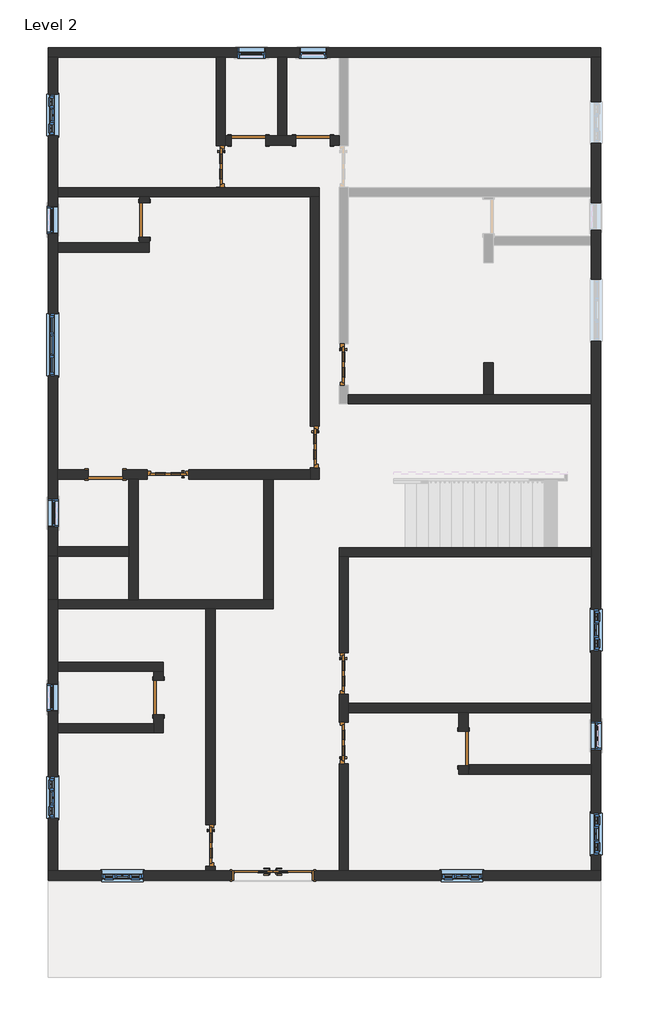
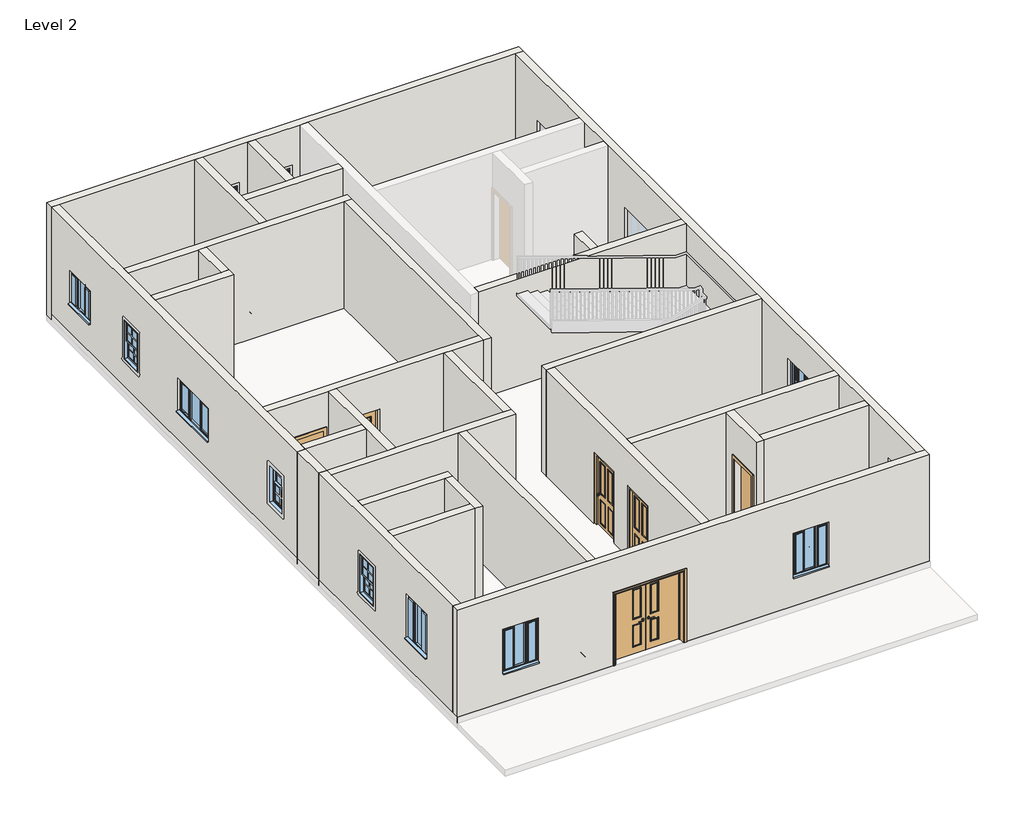
# One storey, part 1 of 3: 29 walls, 14 doors, 13 windows.
"""IFC4 building model written with IfcOpenShell, lengths in millimetres."""

from ifc_helpers import new_model, si_unit, frame, origin, place, context, project, spatial, polyline, outline, extrude, faceted_brep, transform, mapped, element, save
from components import door_2817e3e8, door_51b0c682, doors_intdbl_3_1810x2110mm_301b02ef, doors_intdbl_3_1810x2110mm_13513f6f, door_fadea3f2, door_53b1b562, window_679d2811, windows_tpl_plain_1360x910mm_84993ef1, windows_tpl_w_glazing_cross_bars_910x1210mm_e0b59135, windows_tpl_w_glazing_cross_bars_910x910mm_4aa0f884

model = new_model("IFC4")

# Units and contexts
model_context = context("Model", 3, world=origin())
ifc_project = project(units=[si_unit("LENGTHUNIT", "METRE", prefix="MILLI")], contexts=[model_context])

# Site, building, storey
site = spatial("IfcSite", under=ifc_project)
building = spatial("IfcBuilding", under=site)
storey = spatial("IfcBuildingStorey", under=building, Name="Level 2", Elevation=3048.0)

# Doors
placement = place(None, origin())
door_shape = door_2817e3e8(model_context)
element("IfcDoor", 1, ObjectType="Doors_ExtSgl_2 : 2'x7\"", at=placement, inside=storey, context=model_context, shape_type="MappedRepresentation", body=[
    mapped(door_shape, transform((-2349.4166288, 6357.8803322, 3048.0), x_axis=(0.0, -1.0, 0.0), y_axis=(1.0, 0.0, 0.0), z_axis=(0.0, 0.0, 1.0))),
])
element("IfcDoor", 2, ObjectType="Doors_ExtSgl_2 : 2'x7\"", at=placement, inside=storey, context=model_context, shape_type="MappedRepresentation", body=[
    mapped(door_shape, transform((-286.4451949, 208.0340986, 3048.0), x_axis=(0.0, -1.0, 0.0), y_axis=(1.0, 0.0, 0.0), z_axis=(0.0, 0.0, 1.0))),
])
element("IfcDoor", 3, ObjectType="Doors_ExtSgl_2 : 2'x7\"", at=placement, inside=storey, context=model_context, shape_type="MappedRepresentation", body=[
    mapped(door_shape, transform((348.5548051, -6285.6488489, 3048.0), x_axis=(0.0, 1.0, 0.0), y_axis=(-1.0, 0.0, 0.0), z_axis=(0.0, 0.0, 1.0))),
])
element("IfcDoor", 4, ObjectType="Doors_ExtSgl_2 : 2'x7\"", at=placement, inside=storey, context=model_context, shape_type="MappedRepresentation", body=[
    mapped(door_shape, transform((-2575.1220989, -8536.1734342, 3048.0), x_axis=(0.0, -1.0, 0.0), y_axis=(1.0, 0.0, 0.0), z_axis=(0.0, 0.0, 1.0))),
])
door_2_shape = door_51b0c682(model_context)
element("IfcDoor", 5, ObjectType="Doors_ExtSgl_2 : 2'x7\"", at=placement, inside=storey, context=model_context, shape_type="MappedRepresentation", body=[
    mapped(door_2_shape, transform((348.5548051, -4761.6488489, 3048.0), x_axis=(0.0, -1.0, 0.0), y_axis=(1.0, 0.0, 0.0), z_axis=(0.0, 0.0, 1.0))),
])
element("IfcDoor", 6, ObjectType="Doors_ExtSgl_2 : 2'x7\"", at=placement, inside=storey, context=model_context, shape_type="MappedRepresentation", body=[
    mapped(door_2_shape, transform((-3502.9153286, -401.5659014, 3048.0), x_axis=(-1.0, 0.0, 0.0), y_axis=(0.0, -1.0, 0.0), z_axis=(0.0, 0.0, 1.0))),
])
element("IfcDoor", 7, ObjectType="Doors_ExtSgl_2 : 2'x7\"", at=placement, inside=storey, context=model_context, shape_type="MappedRepresentation", body=[
    mapped(door_2_shape, transform((348.5548051, 2011.4340986, 3048.0), x_axis=(0.0, -1.0, 0.0), y_axis=(1.0, 0.0, 0.0), z_axis=(0.0, 0.0, 1.0))),
])
doors_intdbl_3_1810x2110mm_shape = doors_intdbl_3_1810x2110mm_301b02ef(model_context)
doors_intdbl_3_1810x2110mm_2_shape = doors_intdbl_3_1810x2110mm_13513f6f(model_context)
element("IfcDoor", 8, ObjectType="Doors_IntDbl_3 : 1810x2110mm", at=placement, inside=storey, context=model_context, shape_type="MappedRepresentation", body=[
    mapped(doors_intdbl_3_1810x2110mm_shape, transform((-1203.5220989, -9196.5734342, 3048.0), x_axis=(-1.0, 0.0, 0.0), y_axis=(0.0, -1.0, 0.0), z_axis=(0.0, 0.0, 1.0))),
    mapped(doors_intdbl_3_1810x2110mm_2_shape, transform((-1203.5220989, -9196.5734342, 3048.0), x_axis=(-1.0, 0.0, 0.0), y_axis=(0.0, -1.0, 0.0), z_axis=(0.0, 0.0, 1.0))),
])
door_3_shape = door_fadea3f2(model_context)
element("IfcDoor", 9, ObjectType="Single-Flush : 30\" x 80\"", at=placement, inside=storey, context=model_context, shape_type="MappedRepresentation", body=[
    mapped(door_3_shape, transform((-1739.8166288, 6926.3340986, 3048.0), x_axis=(1.0, 0.0, 0.0), y_axis=(0.0, 1.0, 0.0), z_axis=(0.0, 0.0, 1.0))),
])
element("IfcDoor", 10, ObjectType="Single-Flush : 30\" x 80\"", at=placement, inside=storey, context=model_context, shape_type="MappedRepresentation", body=[
    mapped(door_3_shape, transform((-4874.5153286, -401.5659014, 3048.0), x_axis=(-1.0, 0.0, 0.0), y_axis=(0.0, -1.0, 0.0), z_axis=(0.0, 0.0, 1.0))),
])
door_4_shape = door_53b1b562(model_context)
element("IfcDoor", 11, ObjectType="Single-Flush : 30\" x 80\"", at=placement, inside=storey, context=model_context, shape_type="MappedRepresentation", body=[
    mapped(door_4_shape, transform((-324.5451949, 6926.3340986, 3048.0), x_axis=(-1.0, 0.0, 0.0), y_axis=(0.0, -1.0, 0.0), z_axis=(0.0, 0.0, 1.0))),
])
element("IfcDoor", 12, ObjectType="Single-Flush : 30\" x 80\"", at=placement, inside=storey, context=model_context, shape_type="MappedRepresentation", body=[
    mapped(door_4_shape, transform((-3715.4451949, -5291.0659014, 3048.0), x_axis=(0.0, -1.0, 0.0), y_axis=(1.0, 0.0, 0.0), z_axis=(0.0, 0.0, 1.0))),
])
element("IfcDoor", 13, ObjectType="Single-Flush : 30\" x 80\"", at=placement, inside=storey, context=model_context, shape_type="MappedRepresentation", body=[
    mapped(door_4_shape, transform((2977.4548051, -6412.6488489, 3048.0), x_axis=(0.0, 1.0, 0.0), y_axis=(-1.0, 0.0, 0.0), z_axis=(0.0, 0.0, 1.0))),
])
element("IfcDoor", 14, ObjectType="Single-Flush : 30\" x 80\"", at=placement, inside=storey, context=model_context, shape_type="MappedRepresentation", body=[
    mapped(door_4_shape, transform((-4023.5839448, 5183.1303322, 3048.0), x_axis=(0.0, -1.0, 0.0), y_axis=(1.0, 0.0, 0.0), z_axis=(0.0, 0.0, 1.0))),
])

# Walls
element("IfcWall", 15, ObjectType="Generic - 4.5\" p", at=placement, inside=storey, context=model_context, shape_type="Brep", body=[
    faceted_brep([(-5928.5839448, 5687.8265658, 3048.0), (-4125.1839448, 5687.8265658, 3048.0), (-3921.9839448, 5687.8265658, 3048.0), (-388.0451949, 5687.8265658, 3048.0), (-184.8451949, 5687.8265658, 3048.0), (-184.8451949, 5687.8265658, 6096.0), (-388.0451949, 5687.8265658, 6096.0), (-3921.9839448, 5687.8265658, 6096.0), (-4125.1839448, 5687.8265658, 6096.0), (-5928.5839448, 5687.8265658, 6096.0), (-5928.5839448, 5891.0265658, 3048.0), (-5928.5839448, 5891.0265658, 6096.0), (-2451.0166288, 5891.0265658, 6096.0), (-2247.8166288, 5891.0265658, 6096.0), (-184.8451949, 5891.0265658, 6096.0), (-184.8451949, 5891.0265658, 3048.0), (-2247.8166288, 5891.0265658, 3048.0), (-2451.0166288, 5891.0265658, 3048.0)], [[[0, 1, 2, 3, 4, 5, 6, 7, 8, 9]], [[10, 11, 12, 13, 14, 15, 16, 17]], [[4, 3, 2, 1, 0, 10, 17, 16, 15]], [[0, 9, 11, 10]], [[5, 4, 15, 14]], [[9, 8, 7, 6, 5, 14, 13, 12, 11]]]),
])
element("IfcWall", 16, ObjectType="Generic - 4.5\" p", at=placement, inside=storey, context=model_context, shape_type="Brep", body=[
    faceted_brep([(-388.0451949, -246.9659014, 5158.0), (-388.0451949, -246.9659014, 3048.0), (-388.0451949, -299.9659014, 3048.0), (-388.0451949, -503.1659014, 3048.0), (-388.0451949, -503.1659014, 6096.0), (-388.0451949, -299.9659014, 6096.0), (-388.0451949, 5687.8265658, 6096.0), (-388.0451949, 5687.8265658, 3048.0), (-388.0451949, 663.0340986, 3048.0), (-388.0451949, 663.0340986, 5158.0), (-184.8451949, -503.1659014, 3048.0), (-184.8451949, -246.9659014, 3048.0), (-184.8451949, -246.9659014, 5158.0), (-184.8451949, 663.0340986, 5158.0), (-184.8451949, 663.0340986, 3048.0), (-184.8451949, 5687.8265658, 3048.0), (-184.8451949, 5687.8265658, 6096.0), (-184.8451949, -503.1659014, 6096.0)], [[[0, 1, 2, 3, 4, 5, 6, 7, 8, 9]], [[10, 11, 12, 13, 14, 15, 16, 17]], [[8, 7, 15, 14]], [[3, 2, 1, 11, 10]], [[7, 6, 16, 15]], [[4, 3, 10, 17]], [[14, 13, 9, 8]], [[12, 11, 1, 0]], [[13, 12, 0, 9]], [[6, 5, 4, 17, 16]]]),
])
element("IfcWall", 17, ObjectType="Generic - 4.5\" p", at=placement, inside=storey, context=model_context, shape_type="Brep", body=[
    faceted_brep([(-5255.5153286, -299.9659014, 5080.0), (-5255.5153286, -299.9659014, 3048.0), (-5928.5839448, -299.9659014, 3048.0), (-5928.5839448, -299.9659014, 6096.0), (-388.0451949, -299.9659014, 6096.0), (-388.0451949, -299.9659014, 3048.0), (-3047.9153286, -299.9659014, 3048.0), (-3047.9153286, -299.9659014, 5158.0), (-3957.9153286, -299.9659014, 5158.0), (-3957.9153286, -299.9659014, 3048.0), (-4493.5153286, -299.9659014, 3048.0), (-4493.5153286, -299.9659014, 5080.0), (-5928.5839448, -503.1659014, 3048.0), (-5255.5153286, -503.1659014, 3048.0), (-5255.5153286, -503.1659014, 5080.0), (-4493.5153286, -503.1659014, 5080.0), (-4493.5153286, -503.1659014, 3048.0), (-4366.5153286, -503.1659014, 3048.0), (-4163.3153286, -503.1659014, 3048.0), (-3957.9153286, -503.1659014, 3048.0), (-3957.9153286, -503.1659014, 5158.0), (-3047.9153286, -503.1659014, 5158.0), (-3047.9153286, -503.1659014, 3048.0), (-1404.0451949, -503.1659014, 3048.0), (-1200.8451949, -503.1659014, 3048.0), (-388.0451949, -503.1659014, 3048.0), (-388.0451949, -503.1659014, 6096.0), (-1200.8451949, -503.1659014, 6096.0), (-1404.0451949, -503.1659014, 6096.0), (-4163.3153286, -503.1659014, 6096.0), (-4366.5153286, -503.1659014, 6096.0), (-5928.5839448, -503.1659014, 6096.0)], [[[0, 1, 2, 3, 4, 5, 6, 7, 8, 9, 10, 11]], [[12, 13, 14, 15, 16, 17, 18, 19, 20, 21, 22, 23, 24, 25, 26, 27, 28, 29, 30, 31]], [[6, 5, 25, 24, 23, 22]], [[10, 9, 19, 18, 17, 16]], [[2, 1, 13, 12]], [[5, 4, 26, 25]], [[3, 2, 12, 31]], [[22, 21, 7, 6]], [[20, 19, 9, 8]], [[21, 20, 8, 7]], [[14, 13, 1, 0]], [[15, 14, 0, 11]], [[16, 15, 11, 10]], [[4, 3, 31, 30, 29, 28, 27, 26]]]),
])
element("IfcWall", 18, ObjectType="Generic - 4.5\" p", at=placement, inside=storey, context=model_context, shape_type="Brep", body=[
    faceted_brep([(-4366.5153286, -503.1659014, 3048.0), (-4366.5153286, -1989.0659014, 3048.0), (-4366.5153286, -2192.2659014, 3048.0), (-4366.5153286, -3144.7659014, 3048.0), (-4366.5153286, -3144.7659014, 6096.0), (-4366.5153286, -2192.2659014, 6096.0), (-4366.5153286, -1989.0659014, 6096.0), (-4366.5153286, -503.1659014, 6096.0), (-4163.3153286, -503.1659014, 3048.0), (-4163.3153286, -503.1659014, 6096.0), (-4163.3153286, -3144.7659014, 6096.0), (-4163.3153286, -3144.7659014, 3048.0)], [[[0, 1, 2, 3, 4, 5, 6, 7]], [[8, 9, 10, 11]], [[3, 2, 1, 0, 8, 11]], [[0, 7, 9, 8]], [[4, 3, 11, 10]], [[7, 6, 5, 4, 10, 9]]]),
])
element("IfcWall", 19, ObjectType="Generic - 4.5\" p", at=placement, inside=storey, context=model_context, shape_type="Brep", body=[
    faceted_brep([(-5928.5839448, -3347.9659014, 3048.0), (-2676.7220989, -3347.9659014, 3048.0), (-2473.5220989, -3347.9659014, 3048.0), (-1200.8451949, -3347.9659014, 3048.0), (-1200.8451949, -3347.9659014, 6096.0), (-2473.5220989, -3347.9659014, 6096.0), (-2676.7220989, -3347.9659014, 6096.0), (-5928.5839448, -3347.9659014, 6096.0), (-5928.5839448, -3144.7659014, 3048.0), (-5928.5839448, -3144.7659014, 6096.0), (-4366.5153286, -3144.7659014, 6096.0), (-4163.3153286, -3144.7659014, 6096.0), (-1404.0451949, -3144.7659014, 6096.0), (-1200.8451949, -3144.7659014, 6096.0), (-1200.8451949, -3144.7659014, 3048.0), (-1404.0451949, -3144.7659014, 3048.0), (-4163.3153286, -3144.7659014, 3048.0), (-4366.5153286, -3144.7659014, 3048.0)], [[[0, 1, 2, 3, 4, 5, 6, 7]], [[8, 9, 10, 11, 12, 13, 14, 15, 16, 17]], [[3, 2, 1, 0, 8, 17, 16, 15, 14]], [[0, 7, 9, 8]], [[4, 3, 14, 13]], [[7, 6, 5, 4, 13, 12, 11, 10, 9]]]),
])
element("IfcWall", 20, ObjectType="Generic - 4.5\" p", at=placement, inside=storey, context=model_context, shape_type="SweptSolid", body=[
    extrude(outline(polyline([(-4366.5153286, -2192.2659014), (-5928.5839448, -2192.2659014), (-5928.5839448, -1989.0659014), (-4366.5153286, -1989.0659014), (-4366.5153286, -2192.2659014)])), frame((0.0, 0.0, 3048.0), z_axis=(0.0, 0.0, 1.0), x_axis=(1.0, 0.0, 0.0)), (0.0, 0.0, 1.0), 3048.0),
])
element("IfcWall", 21, ObjectType="Generic - 4.5\" p", at=placement, inside=storey, context=model_context, shape_type="SweptSolid", body=[
    extrude(outline(polyline([(-1404.0451949, -3144.7659014), (-1404.0451949, -503.1659014), (-1200.8451949, -503.1659014), (-1200.8451949, -3144.7659014), (-1404.0451949, -3144.7659014)])), frame((0.0, 0.0, 3048.0), z_axis=(0.0, 0.0, 1.0), x_axis=(1.0, 0.0, 0.0)), (0.0, 0.0, 1.0), 3048.0),
])
element("IfcWall", 22, ObjectType="Generic - 4.5\" p", at=placement, inside=storey, context=model_context, shape_type="Brep", body=[
    faceted_brep([(-5928.5839448, -4719.5659014, 3048.0), (-3817.0451949, -4719.5659014, 3048.0), (-3613.8451949, -4719.5659014, 3048.0), (-3613.8451949, -4719.5659014, 6096.0), (-3817.0451949, -4719.5659014, 6096.0), (-5928.5839448, -4719.5659014, 6096.0), (-5928.5839448, -4516.3659014, 3048.0), (-5928.5839448, -4516.3659014, 6096.0), (-3613.8451949, -4516.3659014, 6096.0), (-3613.8451949, -4516.3659014, 3048.0)], [[[0, 1, 2, 3, 4, 5]], [[6, 7, 8, 9]], [[2, 1, 0, 6, 9]], [[0, 5, 7, 6]], [[3, 2, 9, 8]], [[5, 4, 3, 8, 7]]]),
])
element("IfcWall", 23, ObjectType="Generic - 4.5\" p", at=placement, inside=storey, context=model_context, shape_type="Brep", body=[
    faceted_brep([(-3817.0451949, -5672.0659014, 5080.0), (-3817.0451949, -5672.0659014, 3048.0), (-3817.0451949, -5862.5659014, 3048.0), (-3817.0451949, -6065.7659014, 3048.0), (-3817.0451949, -6065.7659014, 6096.0), (-3817.0451949, -5862.5659014, 6096.0), (-3817.0451949, -4719.5659014, 6096.0), (-3817.0451949, -4719.5659014, 3048.0), (-3817.0451949, -4910.0659014, 3048.0), (-3817.0451949, -4910.0659014, 5080.0), (-3613.8451949, -6065.7659014, 3048.0), (-3613.8451949, -5672.0659014, 3048.0), (-3613.8451949, -5672.0659014, 5080.0), (-3613.8451949, -4910.0659014, 5080.0), (-3613.8451949, -4910.0659014, 3048.0), (-3613.8451949, -4719.5659014, 3048.0), (-3613.8451949, -4719.5659014, 6096.0), (-3613.8451949, -6065.7659014, 6096.0)], [[[0, 1, 2, 3, 4, 5, 6, 7, 8, 9]], [[10, 11, 12, 13, 14, 15, 16, 17]], [[8, 7, 15, 14]], [[3, 2, 1, 11, 10]], [[7, 6, 16, 15]], [[4, 3, 10, 17]], [[12, 11, 1, 0]], [[13, 12, 0, 9]], [[14, 13, 9, 8]], [[6, 5, 4, 17, 16]]]),
])
element("IfcWall", 24, ObjectType="Generic - 4.5\" p", at=placement, inside=storey, context=model_context, shape_type="SweptSolid", body=[
    extrude(outline(polyline([(-5928.5839448, -5862.5659014), (-3817.0451949, -5862.5659014), (-3817.0451949, -6065.7659014), (-5928.5839448, -6065.7659014), (-5928.5839448, -5862.5659014)])), frame((0.0, 0.0, 3048.0), z_axis=(0.0, 0.0, 1.0), x_axis=(1.0, 0.0, 0.0)), (0.0, 0.0, 1.0), 3048.0),
])
element("IfcWall", 25, ObjectType="Generic - 4.5\" p", at=placement, inside=storey, context=model_context, shape_type="SweptSolid", body=[
    extrude(outline(polyline([(-8991.1734342, 5158.0), (-8991.1734342, 3048.0), (-9094.9734342, 3048.0), (-9094.9734342, 6096.0), (-3347.9659014, 6096.0), (-3347.9659014, 3048.0), (-8081.1734342, 3048.0), (-8081.1734342, 5158.0), (-8991.1734342, 5158.0)])), frame((-2676.7220989, 0.0, 0.0), z_axis=(1.0, 0.0, 0.0), x_axis=(0.0, 1.0, 0.0)), (0.0, 0.0, 1.0), 203.2),
])
element("IfcWall", 26, ObjectType="Generic - 4.5\" p", at=placement, inside=storey, context=model_context, shape_type="Brep", body=[
    faceted_brep([(-5928.5839448, 4475.2340986, 3048.0), (-3921.9839448, 4475.2340986, 3048.0), (-3921.9839448, 4475.2340986, 6096.0), (-5928.5839448, 4475.2340986, 6096.0), (-5928.5839448, 4678.4340986, 3048.0), (-5928.5839448, 4678.4340986, 6096.0), (-4125.1839448, 4678.4340986, 6096.0), (-3921.9839448, 4678.4340986, 6096.0), (-3921.9839448, 4678.4340986, 3048.0), (-4125.1839448, 4678.4340986, 3048.0)], [[[0, 1, 2, 3]], [[4, 5, 6, 7, 8, 9]], [[1, 0, 4, 9, 8]], [[0, 3, 5, 4]], [[2, 1, 8, 7]], [[3, 2, 7, 6, 5]]]),
])
element("IfcWall", 27, ObjectType="Generic - 4.5\" p", at=placement, inside=storey, context=model_context, shape_type="SweptSolid", body=[
    extrude(outline(polyline([(4802.1303322, 5080.0), (4802.1303322, 3048.0), (4678.4340986, 3048.0), (4678.4340986, 6096.0), (5687.8265658, 6096.0), (5687.8265658, 3048.0), (5564.1303322, 3048.0), (5564.1303322, 5080.0), (4802.1303322, 5080.0)])), frame((-4125.1839448, 0.0, 0.0), z_axis=(1.0, 0.0, 0.0), x_axis=(0.0, 1.0, 0.0)), (0.0, 0.0, 1.0), 203.2),
])
element("IfcWall", 28, ObjectType="Generic - 4.5\" p", at=placement, inside=storey, context=model_context, shape_type="Brep", body=[
    faceted_brep([(-2451.0166288, 5902.8803322, 5158.0), (-2451.0166288, 5902.8803322, 3048.0), (-2451.0166288, 5891.0265658, 3048.0), (-2451.0166288, 5891.0265658, 6096.0), (-2451.0166288, 8752.5974079, 6096.0), (-2451.0166288, 8752.5974079, 3048.0), (-2451.0166288, 6812.8803322, 3048.0), (-2451.0166288, 6812.8803322, 5158.0), (-2247.8166288, 5891.0265658, 3048.0), (-2247.8166288, 5902.8803322, 3048.0), (-2247.8166288, 5902.8803322, 5158.0), (-2247.8166288, 6812.8803322, 5158.0), (-2247.8166288, 6812.8803322, 3048.0), (-2247.8166288, 6824.7340986, 3048.0), (-2247.8166288, 7027.9340986, 3048.0), (-2247.8166288, 8752.5974079, 3048.0), (-2247.8166288, 8752.5974079, 6096.0), (-2247.8166288, 7027.9340986, 6096.0), (-2247.8166288, 6824.7340986, 6096.0), (-2247.8166288, 5891.0265658, 6096.0)], [[[0, 1, 2, 3, 4, 5, 6, 7]], [[8, 9, 10, 11, 12, 13, 14, 15, 16, 17, 18, 19]], [[6, 5, 15, 14, 13, 12]], [[2, 1, 9, 8]], [[5, 4, 16, 15]], [[3, 2, 8, 19]], [[12, 11, 7, 6]], [[10, 9, 1, 0]], [[11, 10, 0, 7]], [[4, 3, 19, 18, 17, 16]]]),
])
element("IfcWall", 29, ObjectType="Generic - 4.5\" p", at=placement, inside=storey, context=model_context, shape_type="Brep", body=[
    faceted_brep([(-1358.8166288, 6824.7340986, 3048.0), (-705.5451949, 6824.7340986, 3048.0), (-705.5451949, 6824.7340986, 5080.0), (56.4548051, 6824.7340986, 5080.0), (56.4548051, 6824.7340986, 3048.0), (246.9548051, 6824.7340986, 3048.0), (246.9548051, 6824.7340986, 6096.0), (-2247.8166288, 6824.7340986, 6096.0), (-2247.8166288, 6824.7340986, 3048.0), (-2120.8166288, 6824.7340986, 3048.0), (-2120.8166288, 6824.7340986, 5080.0), (-1358.8166288, 6824.7340986, 5080.0), (-705.5451949, 7027.9340986, 5080.0), (-705.5451949, 7027.9340986, 3048.0), (-896.0451949, 7027.9340986, 3048.0), (-1099.2451949, 7027.9340986, 3048.0), (-1358.8166288, 7027.9340986, 3048.0), (-1358.8166288, 7027.9340986, 5080.0), (-2120.8166288, 7027.9340986, 5080.0), (-2120.8166288, 7027.9340986, 3048.0), (-2247.8166288, 7027.9340986, 3048.0), (-2247.8166288, 7027.9340986, 6096.0), (-1099.2451949, 7027.9340986, 6096.0), (-896.0451949, 7027.9340986, 6096.0), (246.9548051, 7027.9340986, 6096.0), (246.9548051, 7027.9340986, 3048.0), (56.4548051, 7027.9340986, 3048.0), (56.4548051, 7027.9340986, 5080.0)], [[[0, 1, 2, 3, 4, 5, 6, 7, 8, 9, 10, 11]], [[12, 13, 14, 15, 16, 17, 18, 19, 20, 21, 22, 23, 24, 25, 26, 27]], [[9, 8, 20, 19]], [[26, 25, 5, 4]], [[16, 15, 14, 13, 1, 0]], [[8, 7, 21, 20]], [[6, 5, 25, 24]], [[17, 16, 0, 11]], [[18, 17, 11, 10]], [[19, 18, 10, 9]], [[2, 1, 13, 12]], [[3, 2, 12, 27]], [[4, 3, 27, 26]], [[7, 6, 24, 23, 22, 21]]]),
])
element("IfcWall", 30, ObjectType="Generic - 4.5\" p", at=placement, inside=storey, context=model_context, shape_type="SweptSolid", body=[
    extrude(outline(polyline([(-1099.2451949, 7027.9340986), (-1099.2451949, 8752.5974079), (-896.0451949, 8752.5974079), (-896.0451949, 7027.9340986), (-1099.2451949, 7027.9340986)])), frame((0.0, 0.0, 3048.0), z_axis=(0.0, 0.0, 1.0), x_axis=(1.0, 0.0, 0.0)), (0.0, 0.0, 1.0), 3048.0),
])
element("IfcWall", 31, ObjectType="Generic - 4.5\" p", at=placement, inside=storey, context=model_context, shape_type="Brep", body=[
    faceted_brep([(450.1548051, 1147.8340986, 3048.0), (5778.5439795, 1147.8340986, 3048.0), (5778.5439795, 1147.8340986, 6096.0), (450.1548051, 1147.8340986, 6096.0), (450.1548051, 1351.0340986, 3048.0), (450.1548051, 1351.0340986, 6096.0), (3421.9548051, 1351.0340986, 6096.0), (3625.1548051, 1351.0340986, 6096.0), (5778.5439795, 1351.0340986, 6096.0), (5778.5439795, 1351.0340986, 3048.0), (3625.1548051, 1351.0340986, 3048.0), (3421.9548051, 1351.0340986, 3048.0)], [[[0, 1, 2, 3]], [[4, 5, 6, 7, 8, 9, 10, 11]], [[1, 0, 4, 11, 10, 9]], [[0, 3, 5, 4]], [[2, 1, 9, 8]], [[3, 2, 8, 7, 6, 5]]]),
])
element("IfcWall", 32, ObjectType="Generic - 4.5\" p", at=placement, inside=storey, context=model_context, shape_type="SweptSolid", body=[
    extrude(outline(polyline([(3625.1548051, 2047.4361958), (3625.1548051, 1351.0340986), (3421.9548051, 1351.0340986), (3421.9548051, 2047.4361958), (3625.1548051, 2047.4361958)])), frame((0.0, 0.0, 3048.0), z_axis=(0.0, 0.0, 1.0), x_axis=(1.0, 0.0, 0.0)), (0.0, 0.0, 1.0), 3048.0),
])
element("IfcWall", 33, ObjectType="Generic - 4.5\" p", at=placement, inside=storey, context=model_context, shape_type="Brep", body=[
    faceted_brep([(5778.5439795, -2004.8977001, 3048.0), (246.9548051, -2004.8977001, 3048.0), (246.9548051, -2004.8977001, 6096.0), (5778.5439795, -2004.8977001, 6096.0), (5778.5439795, -2208.0977001, 3048.0), (5778.5439795, -2208.0977001, 6096.0), (450.1548051, -2208.0977001, 6096.0), (246.9548051, -2208.0977001, 6096.0), (246.9548051, -2208.0977001, 3048.0), (450.1548051, -2208.0977001, 3048.0)], [[[0, 1, 2, 3]], [[4, 5, 6, 7, 8, 9]], [[1, 0, 4, 9, 8]], [[0, 3, 5, 4]], [[2, 1, 8, 7]], [[3, 2, 7, 6, 5]]]),
])
element("IfcWall", 34, ObjectType="Generic - 4.5\" p", at=placement, inside=storey, context=model_context, shape_type="Brep", body=[
    faceted_brep([(246.9548051, -5216.6488489, 3048.0), (246.9548051, -5830.6488489, 3048.0), (246.9548051, -5830.6488489, 5158.0), (246.9548051, -6740.6488489, 5158.0), (246.9548051, -6740.6488489, 3048.0), (246.9548051, -9094.9734342, 3048.0), (246.9548051, -9094.9734342, 6096.0), (246.9548051, -2208.0977001, 6096.0), (246.9548051, -2208.0977001, 3048.0), (246.9548051, -4306.6488489, 3048.0), (246.9548051, -4306.6488489, 5158.0), (246.9548051, -5216.6488489, 5158.0), (450.1548051, -5830.6488489, 5158.0), (450.1548051, -5830.6488489, 3048.0), (450.1548051, -5625.2488489, 3048.0), (450.1548051, -5422.0488489, 3048.0), (450.1548051, -5216.6488489, 3048.0), (450.1548051, -5216.6488489, 5158.0), (450.1548051, -4306.6488489, 5158.0), (450.1548051, -4306.6488489, 3048.0), (450.1548051, -2208.0977001, 3048.0), (450.1548051, -2208.0977001, 6096.0), (450.1548051, -5422.0488489, 6096.0), (450.1548051, -5625.2488489, 6096.0), (450.1548051, -9094.9734342, 6096.0), (450.1548051, -9094.9734342, 3048.0), (450.1548051, -6740.6488489, 3048.0), (450.1548051, -6740.6488489, 5158.0)], [[[0, 1, 2, 3, 4, 5, 6, 7, 8, 9, 10, 11]], [[12, 13, 14, 15, 16, 17, 18, 19, 20, 21, 22, 23, 24, 25, 26, 27]], [[9, 8, 20, 19]], [[26, 25, 5, 4]], [[16, 15, 14, 13, 1, 0]], [[8, 7, 21, 20]], [[6, 5, 25, 24]], [[19, 18, 10, 9]], [[17, 16, 0, 11]], [[18, 17, 11, 10]], [[4, 3, 27, 26]], [[2, 1, 13, 12]], [[3, 2, 12, 27]], [[7, 6, 24, 23, 22, 21]]]),
])
element("IfcWall", 35, ObjectType="Generic - 4.5\" p", at=placement, inside=storey, context=model_context, shape_type="Brep", body=[
    faceted_brep([(450.1548051, -5625.2488489, 3048.0), (2875.8548051, -5625.2488489, 3048.0), (3079.0548051, -5625.2488489, 3048.0), (5778.5439795, -5625.2488489, 3048.0), (5778.5439795, -5625.2488489, 6096.0), (3079.0548051, -5625.2488489, 6096.0), (2875.8548051, -5625.2488489, 6096.0), (450.1548051, -5625.2488489, 6096.0), (450.1548051, -5422.0488489, 3048.0), (450.1548051, -5422.0488489, 6096.0), (5778.5439795, -5422.0488489, 6096.0), (5778.5439795, -5422.0488489, 3048.0)], [[[0, 1, 2, 3, 4, 5, 6, 7]], [[8, 9, 10, 11]], [[3, 2, 1, 0, 8, 11]], [[4, 3, 11, 10]], [[0, 7, 9, 8]], [[7, 6, 5, 4, 10, 9]]]),
])
element("IfcWall", 36, ObjectType="Generic - 4.5\" p", at=placement, inside=storey, context=model_context, shape_type="Brep", body=[
    faceted_brep([(2875.8548051, -5625.2488489, 3048.0), (2875.8548051, -6031.6488489, 3048.0), (2875.8548051, -6031.6488489, 5080.0), (2875.8548051, -6793.6488489, 5080.0), (2875.8548051, -6793.6488489, 3048.0), (2875.8548051, -6971.4488489, 3048.0), (2875.8548051, -6971.4488489, 6096.0), (2875.8548051, -5625.2488489, 6096.0), (3079.0548051, -6031.6488489, 5080.0), (3079.0548051, -6031.6488489, 3048.0), (3079.0548051, -5625.2488489, 3048.0), (3079.0548051, -5625.2488489, 6096.0), (3079.0548051, -6768.2488489, 6096.0), (3079.0548051, -6971.4488489, 6096.0), (3079.0548051, -6971.4488489, 3048.0), (3079.0548051, -6793.6488489, 3048.0), (3079.0548051, -6793.6488489, 5080.0)], [[[0, 1, 2, 3, 4, 5, 6, 7]], [[8, 9, 10, 11, 12, 13, 14, 15, 16]], [[10, 9, 1, 0]], [[15, 14, 5, 4]], [[0, 7, 11, 10]], [[6, 5, 14, 13]], [[2, 1, 9, 8]], [[3, 2, 8, 16]], [[4, 3, 16, 15]], [[7, 6, 13, 12, 11]]]),
])
element("IfcWall", 37, ObjectType="Generic - 4.5\" p", at=placement, inside=storey, context=model_context, shape_type="SweptSolid", body=[
    extrude(outline(polyline([(3079.0548051, -6768.2488489), (5778.5439795, -6768.2488489), (5778.5439795, -6971.4488489), (3079.0548051, -6971.4488489), (3079.0548051, -6768.2488489)])), frame((0.0, 0.0, 3048.0), z_axis=(0.0, 0.0, 1.0), x_axis=(1.0, 0.0, 0.0)), (0.0, 0.0, 1.0), 3048.0),
])
element("IfcWall", 38, ObjectType="Generic - 4.5\" p", at=placement, inside=storey, context=model_context, shape_type="SweptSolid", body=[
    extrude(outline(polyline([(-6131.7839448, -3144.7659014), (-6131.7839448, -2192.2659014), (-5928.5839448, -2192.2659014), (-5928.5839448, -3144.7659014), (-6131.7839448, -3144.7659014)])), frame((0.0, 0.0, 3048.0), z_axis=(0.0, 0.0, 1.0), x_axis=(1.0, 0.0, 0.0)), (0.0, 0.0, 1.0), 3048.0),
])
element("IfcWall", 39, ObjectType="Generic - 9\" w", at=placement, inside=storey, context=model_context, shape_type="Brep", body=[
    faceted_brep([(-6134.0560205, 8752.5974079, 3048.0), (-6131.7839448, 8752.5974079, 3048.0), (-5928.5839448, 8752.5974079, 3048.0), (-2451.0166288, 8752.5974079, 3048.0), (-2247.8166288, 8752.5974079, 3048.0), (-1099.2451949, 8752.5974079, 3048.0), (-896.0451949, 8752.5974079, 3048.0), (246.9548051, 8752.5974079, 3048.0), (450.1548051, 8752.5974079, 3048.0), (5778.5439795, 8752.5974079, 3048.0), (5981.7439795, 8752.5974079, 3048.0), (5981.7439795, 8752.5974079, 6096.0), (5778.5439795, 8752.5974079, 6096.0), (450.1548051, 8752.5974079, 6096.0), (246.9548051, 8752.5974079, 6096.0), (-896.0451949, 8752.5974079, 6096.0), (-1099.2451949, 8752.5974079, 6096.0), (-2247.8166288, 8752.5974079, 6096.0), (-2451.0166288, 8752.5974079, 6096.0), (-5928.5839448, 8752.5974079, 6096.0), (-6131.7839448, 8752.5974079, 6096.0), (-6134.0560205, 8752.5974079, 6096.0), (-1368.7309118, 8752.5974079, 5029.2), (-1368.7309118, 8752.5974079, 3962.4), (-1978.3309118, 8752.5974079, 3962.4), (-1978.3309118, 8752.5974079, 5029.2), (-19.7451949, 8752.5974079, 5029.2), (-19.7451949, 8752.5974079, 3962.4), (-629.3451949, 8752.5974079, 3962.4), (-629.3451949, 8752.5974079, 5029.2), (-6134.0560205, 8955.7974079, 3048.0), (-6134.0560205, 8955.7974079, 6096.0), (5981.7439795, 8955.7974079, 6096.0), (5981.7439795, 8955.7974079, 3048.0), (-1368.7309118, 8955.7974079, 5029.2), (-1978.3309118, 8955.7974079, 5029.2), (-1978.3309118, 8955.7974079, 3962.4), (-1368.7309118, 8955.7974079, 3962.4), (-19.7451949, 8955.7974079, 5029.2), (-629.3451949, 8955.7974079, 5029.2), (-629.3451949, 8955.7974079, 3962.4), (-19.7451949, 8955.7974079, 3962.4)], [[[0, 1, 2, 3, 4, 5, 6, 7, 8, 9, 10, 11, 12, 13, 14, 15, 16, 17, 18, 19, 20, 21], [22, 23, 24, 25], [26, 27, 28, 29]], [[30, 31, 32, 33], [34, 35, 36, 37], [38, 39, 40, 41]], [[10, 9, 8, 7, 6, 5, 4, 3, 2, 1, 0, 30, 33]], [[0, 21, 31, 30]], [[11, 10, 33, 32]], [[23, 22, 34, 37]], [[24, 23, 37, 36]], [[25, 24, 36, 35]], [[22, 25, 35, 34]], [[27, 26, 38, 41]], [[28, 27, 41, 40]], [[29, 28, 40, 39]], [[26, 29, 39, 38]], [[21, 20, 19, 18, 17, 16, 15, 14, 13, 12, 11, 32, 31]]]),
])
element("IfcWall", 40, ObjectType="Generic - 9\" w", at=placement, inside=storey, context=model_context, shape_type="Brep", body=[
    faceted_brep([(5981.7439795, -9094.9734342, 6096.0), (5981.7439795, -9094.9734342, 3048.0), (5778.5439795, -9094.9734342, 3048.0), (450.1548051, -9094.9734342, 3048.0), (246.9548051, -9094.9734342, 3048.0), (-298.5220989, -9094.9734342, 3048.0), (-298.5220989, -9094.9734342, 5158.0), (-2108.5220989, -9094.9734342, 5158.0), (-2108.5220989, -9094.9734342, 3048.0), (-2473.5220989, -9094.9734342, 3048.0), (-2676.7220989, -9094.9734342, 3048.0), (-5928.5839448, -9094.9734342, 3048.0), (-6131.7839448, -9094.9734342, 3048.0), (-6131.7839448, -9094.9734342, 6096.0), (-5928.5839448, -9094.9734342, 6096.0), (-2676.7220989, -9094.9734342, 6096.0), (-2473.5220989, -9094.9734342, 6096.0), (246.9548051, -9094.9734342, 6096.0), (450.1548051, -9094.9734342, 6096.0), (5778.5439795, -9094.9734342, 6096.0), (3394.3548051, -9094.9734342, 5172.4), (2484.3548051, -9094.9734342, 5172.4), (2484.3548051, -9094.9734342, 3962.4), (3394.3548051, -9094.9734342, 3962.4), (-4051.1839448, -9094.9734342, 5172.4), (-4961.1839448, -9094.9734342, 5172.4), (-4961.1839448, -9094.9734342, 3962.4), (-4051.1839448, -9094.9734342, 3962.4), (5981.7439795, -9298.1734342, 3048.0), (5981.7439795, -9298.1734342, 6096.0), (-6131.7839448, -9298.1734342, 6096.0), (-6131.7839448, -9298.1734342, 3048.0), (-2108.5220989, -9298.1734342, 3048.0), (-2108.5220989, -9298.1734342, 5158.0), (-298.5220989, -9298.1734342, 5158.0), (-298.5220989, -9298.1734342, 3048.0), (3394.3548051, -9298.1734342, 5172.4), (3394.3548051, -9298.1734342, 3962.4), (2484.3548051, -9298.1734342, 3962.4), (2484.3548051, -9298.1734342, 5172.4), (-4051.1839448, -9298.1734342, 5172.4), (-4051.1839448, -9298.1734342, 3962.4), (-4961.1839448, -9298.1734342, 3962.4), (-4961.1839448, -9298.1734342, 5172.4)], [[[0, 1, 2, 3, 4, 5, 6, 7, 8, 9, 10, 11, 12, 13, 14, 15, 16, 17, 18, 19], [20, 21, 22, 23], [24, 25, 26, 27]], [[28, 29, 30, 31, 32, 33, 34, 35], [36, 37, 38, 39], [40, 41, 42, 43]], [[1, 28, 35, 5, 4, 3, 2]], [[31, 12, 11, 10, 9, 8, 32]], [[1, 0, 29, 28]], [[13, 12, 31, 30]], [[7, 33, 32, 8]], [[33, 7, 6, 34]], [[34, 6, 5, 35]], [[37, 36, 20, 23]], [[38, 37, 23, 22]], [[39, 38, 22, 21]], [[36, 39, 21, 20]], [[41, 40, 24, 27]], [[42, 41, 27, 26]], [[43, 42, 26, 25]], [[40, 43, 25, 24]], [[0, 19, 18, 17, 16, 15, 14, 13, 30, 29]]]),
])
element("IfcWall", 41, ObjectType="Generic - 9\" w", at=placement, inside=storey, context=model_context, shape_type="Brep", body=[
    faceted_brep([(-5928.5839448, -9094.9734342, 3048.0), (-5928.5839448, -6065.7659014, 3048.0), (-5928.5839448, -5862.5659014, 3048.0), (-5928.5839448, -4719.5659014, 3048.0), (-5928.5839448, -4516.3659014, 3048.0), (-5928.5839448, -3347.9659014, 3048.0), (-5928.5839448, -3144.7659014, 3048.0), (-5928.5839448, -3144.7659014, 6096.0), (-5928.5839448, -3347.9659014, 6096.0), (-5928.5839448, -4516.3659014, 6096.0), (-5928.5839448, -4719.5659014, 6096.0), (-5928.5839448, -5862.5659014, 6096.0), (-5928.5839448, -6065.7659014, 6096.0), (-5928.5839448, -9094.9734342, 6096.0), (-5928.5839448, -7943.1659014, 5172.4), (-5928.5839448, -7033.1659014, 5172.4), (-5928.5839448, -7033.1659014, 3962.4), (-5928.5839448, -7943.1659014, 3962.4), (-5928.5839448, -5595.8659014, 5029.2), (-5928.5839448, -4986.2659014, 5029.2), (-5928.5839448, -4986.2659014, 3962.4), (-5928.5839448, -5595.8659014, 3962.4), (-6131.7839448, -9094.9734342, 3048.0), (-6131.7839448, -9094.9734342, 6096.0), (-6131.7839448, -3144.7659014, 6096.0), (-6131.7839448, -3144.7659014, 3048.0), (-6131.7839448, -7943.1659014, 5172.4), (-6131.7839448, -7943.1659014, 3962.4), (-6131.7839448, -7033.1659014, 3962.4), (-6131.7839448, -7033.1659014, 5172.4), (-6131.7839448, -5595.8659014, 5029.2), (-6131.7839448, -5595.8659014, 3962.4), (-6131.7839448, -4986.2659014, 3962.4), (-6131.7839448, -4986.2659014, 5029.2)], [[[0, 1, 2, 3, 4, 5, 6, 7, 8, 9, 10, 11, 12, 13], [14, 15, 16, 17], [18, 19, 20, 21]], [[22, 23, 24, 25], [26, 27, 28, 29], [30, 31, 32, 33]], [[6, 5, 4, 3, 2, 1, 0, 22, 25]], [[0, 13, 23, 22]], [[7, 6, 25, 24]], [[27, 26, 14, 17]], [[28, 27, 17, 16]], [[29, 28, 16, 15]], [[26, 29, 15, 14]], [[31, 30, 18, 21]], [[32, 31, 21, 20]], [[33, 32, 20, 19]], [[30, 33, 19, 18]], [[13, 12, 11, 10, 9, 8, 7, 24, 23]]]),
])
element("IfcWall", 42, ObjectType="Generic - 9\" w", at=placement, inside=storey, context=model_context, shape_type="Brep", body=[
    faceted_brep([(-5928.5839448, -2192.2659014, 3048.0), (-5928.5839448, -1989.0659014, 3048.0), (-5928.5839448, -503.1659014, 3048.0), (-5928.5839448, -299.9659014, 3048.0), (-5928.5839448, 4475.2340986, 3048.0), (-5928.5839448, 4678.4340986, 3048.0), (-5928.5839448, 5687.8265658, 3048.0), (-5928.5839448, 5891.0265658, 3048.0), (-5928.5839448, 8752.5974079, 3048.0), (-5928.5839448, 8752.5974079, 6096.0), (-5928.5839448, 5891.0265658, 6096.0), (-5928.5839448, 5687.8265658, 6096.0), (-5928.5839448, 4678.4340986, 6096.0), (-5928.5839448, 4475.2340986, 6096.0), (-5928.5839448, -299.9659014, 6096.0), (-5928.5839448, -503.1659014, 6096.0), (-5928.5839448, -1989.0659014, 6096.0), (-5928.5839448, -2192.2659014, 6096.0), (-5928.5839448, 1763.2340986, 4872.4), (-5928.5839448, 3123.2340986, 4872.4), (-5928.5839448, 3123.2340986, 3962.4), (-5928.5839448, 1763.2340986, 3962.4), (-5928.5839448, 7027.5974079, 4872.4), (-5928.5839448, 7937.5974079, 4872.4), (-5928.5839448, 7937.5974079, 3962.4), (-5928.5839448, 7027.5974079, 3962.4), (-5928.5839448, 4878.3303322, 5029.2), (-5928.5839448, 5487.9303322, 5029.2), (-5928.5839448, 5487.9303322, 3962.4), (-5928.5839448, 4878.3303322, 3962.4), (-5928.5839448, -941.3159014, 5029.2), (-5928.5839448, -941.3159014, 3962.4), (-5928.5839448, -1550.9159014, 3962.4), (-5928.5839448, -1550.9159014, 5029.2), (-6131.7839448, -2192.2659014, 3048.0), (-6131.7839448, -2192.2659014, 6096.0), (-6131.7839448, 8752.5974079, 6096.0), (-6131.7839448, 8752.5974079, 3048.0), (-6131.7839448, 1763.2340986, 4872.4), (-6131.7839448, 1763.2340986, 3962.4), (-6131.7839448, 3123.2340986, 3962.4), (-6131.7839448, 3123.2340986, 4872.4), (-6131.7839448, 7027.5974079, 4872.4), (-6131.7839448, 7027.5974079, 3962.4), (-6131.7839448, 7937.5974079, 3962.4), (-6131.7839448, 7937.5974079, 4872.4), (-6131.7839448, 4878.3303322, 5029.2), (-6131.7839448, 4878.3303322, 3962.4), (-6131.7839448, 5487.9303322, 3962.4), (-6131.7839448, 5487.9303322, 5029.2), (-6131.7839448, -941.3159014, 5029.2), (-6131.7839448, -1550.9159014, 5029.2), (-6131.7839448, -1550.9159014, 3962.4), (-6131.7839448, -941.3159014, 3962.4)], [[[0, 1, 2, 3, 4, 5, 6, 7, 8, 9, 10, 11, 12, 13, 14, 15, 16, 17], [18, 19, 20, 21], [22, 23, 24, 25], [26, 27, 28, 29], [30, 31, 32, 33]], [[34, 35, 36, 37], [38, 39, 40, 41], [42, 43, 44, 45], [46, 47, 48, 49], [50, 51, 52, 53]], [[8, 7, 6, 5, 4, 3, 2, 1, 0, 34, 37]], [[9, 8, 37, 36]], [[0, 17, 35, 34]], [[39, 38, 18, 21]], [[40, 39, 21, 20]], [[41, 40, 20, 19]], [[38, 41, 19, 18]], [[43, 42, 22, 25]], [[44, 43, 25, 24]], [[45, 44, 24, 23]], [[42, 45, 23, 22]], [[47, 46, 26, 29]], [[48, 47, 29, 28]], [[49, 48, 28, 27]], [[46, 49, 27, 26]], [[31, 30, 50, 53]], [[32, 31, 53, 52]], [[33, 32, 52, 51]], [[30, 33, 51, 50]], [[17, 16, 15, 14, 13, 12, 11, 10, 9, 36, 35]]]),
])
element("IfcWall", 43, ObjectType="Generic - 9\" w", at=placement, inside=storey, context=model_context, shape_type="Brep", body=[
    faceted_brep([(5778.5439795, 8752.5974079, 3048.0), (5778.5439795, 5891.0265658, 3048.0), (5778.5439795, 5687.8265658, 3048.0), (5778.5439795, 4830.8340986, 3048.0), (5778.5439795, 4627.6340986, 3048.0), (5778.5439795, 1351.0340986, 3048.0), (5778.5439795, 1147.8340986, 3048.0), (5778.5439795, -2004.8977001, 3048.0), (5778.5439795, -2208.0977001, 3048.0), (5778.5439795, -5422.0488489, 3048.0), (5778.5439795, -5625.2488489, 3048.0), (5778.5439795, -6768.2488489, 3048.0), (5778.5439795, -6971.4488489, 3048.0), (5778.5439795, -9094.9734342, 3048.0), (5778.5439795, -9094.9734342, 6096.0), (5778.5439795, -6971.4488489, 6096.0), (5778.5439795, -6768.2488489, 6096.0), (5778.5439795, -5625.2488489, 6096.0), (5778.5439795, -5422.0488489, 6096.0), (5778.5439795, -2208.0977001, 6096.0), (5778.5439795, -2004.8977001, 6096.0), (5778.5439795, 1147.8340986, 6096.0), (5778.5439795, 1351.0340986, 6096.0), (5778.5439795, 4627.6340986, 6096.0), (5778.5439795, 4830.8340986, 6096.0), (5778.5439795, 5687.8265658, 6096.0), (5778.5439795, 5891.0265658, 6096.0), (5778.5439795, 8752.5974079, 6096.0), (5778.5439795, -7827.1734342, 5172.4), (5778.5439795, -8737.1734342, 5172.4), (5778.5439795, -8737.1734342, 3962.4), (5778.5439795, -7827.1734342, 3962.4), (5778.5439795, -3360.0732745, 5172.4), (5778.5439795, -4270.0732745, 5172.4), (5778.5439795, -4270.0732745, 3962.4), (5778.5439795, -3360.0732745, 3962.4), (5778.5439795, 3885.2340986, 4872.4), (5778.5439795, 2525.2340986, 4872.4), (5778.5439795, 2525.2340986, 3962.4), (5778.5439795, 3885.2340986, 3962.4), (5778.5439795, 7776.8119869, 4872.4), (5778.5439795, 6866.8119869, 4872.4), (5778.5439795, 6866.8119869, 3962.4), (5778.5439795, 7776.8119869, 3962.4), (5778.5439795, 4954.5303322, 5029.2), (5778.5439795, 4954.5303322, 3962.4), (5778.5439795, 5564.1303322, 3962.4), (5778.5439795, 5564.1303322, 5029.2), (5778.5439795, -5828.4488489, 5029.2), (5778.5439795, -6438.0488489, 5029.2), (5778.5439795, -6438.0488489, 3962.4), (5778.5439795, -5828.4488489, 3962.4), (5981.7439795, 8752.5974079, 3048.0), (5981.7439795, 8752.5974079, 6096.0), (5981.7439795, -9094.9734342, 6096.0), (5981.7439795, -9094.9734342, 3048.0), (5981.7439795, -7827.1734342, 5172.4), (5981.7439795, -7827.1734342, 3962.4), (5981.7439795, -8737.1734342, 3962.4), (5981.7439795, -8737.1734342, 5172.4), (5981.7439795, -3360.0732745, 5172.4), (5981.7439795, -3360.0732745, 3962.4), (5981.7439795, -4270.0732745, 3962.4), (5981.7439795, -4270.0732745, 5172.4), (5981.7439795, 3885.2340986, 4872.4), (5981.7439795, 3885.2340986, 3962.4), (5981.7439795, 2525.2340986, 3962.4), (5981.7439795, 2525.2340986, 4872.4), (5981.7439795, 7776.8119869, 4872.4), (5981.7439795, 7776.8119869, 3962.4), (5981.7439795, 6866.8119869, 3962.4), (5981.7439795, 6866.8119869, 4872.4), (5981.7439795, 4954.5303322, 5029.2), (5981.7439795, 5564.1303322, 5029.2), (5981.7439795, 5564.1303322, 3962.4), (5981.7439795, 4954.5303322, 3962.4), (5981.7439795, -5828.4488489, 5029.2), (5981.7439795, -5828.4488489, 3962.4), (5981.7439795, -6438.0488489, 3962.4), (5981.7439795, -6438.0488489, 5029.2)], [[[0, 1, 2, 3, 4, 5, 6, 7, 8, 9, 10, 11, 12, 13, 14, 15, 16, 17, 18, 19, 20, 21, 22, 23, 24, 25, 26, 27], [28, 29, 30, 31], [32, 33, 34, 35], [36, 37, 38, 39], [40, 41, 42, 43], [44, 45, 46, 47], [48, 49, 50, 51]], [[52, 53, 54, 55], [56, 57, 58, 59], [60, 61, 62, 63], [64, 65, 66, 67], [68, 69, 70, 71], [72, 73, 74, 75], [76, 77, 78, 79]], [[13, 12, 11, 10, 9, 8, 7, 6, 5, 4, 3, 2, 1, 0, 52, 55]], [[0, 27, 53, 52]], [[14, 13, 55, 54]], [[57, 56, 28, 31]], [[58, 57, 31, 30]], [[59, 58, 30, 29]], [[56, 59, 29, 28]], [[61, 60, 32, 35]], [[62, 61, 35, 34]], [[63, 62, 34, 33]], [[60, 63, 33, 32]], [[65, 64, 36, 39]], [[66, 65, 39, 38]], [[67, 66, 38, 37]], [[64, 67, 37, 36]], [[69, 68, 40, 43]], [[70, 69, 43, 42]], [[71, 70, 42, 41]], [[68, 71, 41, 40]], [[45, 44, 72, 75]], [[46, 45, 75, 74]], [[47, 46, 74, 73]], [[44, 47, 73, 72]], [[77, 76, 48, 51]], [[78, 77, 51, 50]], [[79, 78, 50, 49]], [[76, 79, 49, 48]], [[27, 26, 25, 24, 23, 22, 21, 20, 19, 18, 17, 16, 15, 14, 54, 53]]]),
])

# Windows
window_shape = window_679d2811(model_context)
element("IfcWindow", 44, ObjectType="Window-Double-Hung : 24\" x 42\"", at=placement, inside=storey, context=model_context, shape_type="MappedRepresentation", body=[
    mapped(window_shape, transform((-6030.1839448, 5183.1303322, 3048.0), x_axis=(0.0, 1.0, 0.0), y_axis=(-1.0, 0.0, 0.0), z_axis=(0.0, 0.0, 1.0))),
])
element("IfcWindow", 45, ObjectType="Window-Double-Hung : 24\" x 42\"", at=placement, inside=storey, context=model_context, shape_type="MappedRepresentation", body=[
    mapped(window_shape, transform((-1673.5309118, 8854.1974079, 3048.0), x_axis=(-1.0, 0.0, 0.0), y_axis=(0.0, -1.0, 0.0), z_axis=(0.0, 0.0, 1.0))),
])
element("IfcWindow", 46, ObjectType="Window-Double-Hung : 24\" x 42\"", at=placement, inside=storey, context=model_context, shape_type="MappedRepresentation", body=[
    mapped(window_shape, transform((-324.5451949, 8854.1974079, 3048.0), x_axis=(-1.0, 0.0, 0.0), y_axis=(0.0, -1.0, 0.0), z_axis=(0.0, 0.0, 1.0))),
])
element("IfcWindow", 47, ObjectType="Window-Double-Hung : 24\" x 42\"", at=placement, inside=storey, context=model_context, shape_type="MappedRepresentation", body=[
    mapped(window_shape, transform((5880.1439795, -6133.2488489, 3048.0), x_axis=(0.0, -1.0, 0.0), y_axis=(1.0, 0.0, 0.0), z_axis=(0.0, 0.0, 1.0))),
])
element("IfcWindow", 48, ObjectType="Window-Double-Hung : 24\" x 42\"", at=placement, inside=storey, context=model_context, shape_type="MappedRepresentation", body=[
    mapped(window_shape, transform((-6030.1839448, -5291.0659014, 3048.0), x_axis=(0.0, 1.0, 0.0), y_axis=(-1.0, 0.0, 0.0), z_axis=(0.0, 0.0, 1.0))),
])
element("IfcWindow", 49, ObjectType="Window-Double-Hung : 24\" x 42\"", at=placement, inside=storey, context=model_context, shape_type="MappedRepresentation", body=[
    mapped(window_shape, transform((-6030.1839448, -1246.1159014, 3048.0), x_axis=(0.0, -1.0, 0.0), y_axis=(1.0, 0.0, 0.0), z_axis=(0.0, 0.0, 1.0))),
])
windows_tpl_plain_1360x910mm_shape = windows_tpl_plain_1360x910mm_84993ef1(model_context)
element("IfcWindow", 50, ObjectType="Windows_Tpl_Plain : 1360x910mm", at=placement, inside=storey, context=model_context, shape_type="MappedRepresentation", body=[
    mapped(windows_tpl_plain_1360x910mm_shape, transform((-6021.727377, 2944.9007653, 2762.4), x_axis=(0.0, 1.0, 0.0), y_axis=(-1.0, 0.0, 0.0), z_axis=(0.0, 0.0, 1.0))),
])
windows_tpl_w_glazing_cross_bars_910x1210mm_shape = windows_tpl_w_glazing_cross_bars_910x1210mm_e0b59135(model_context)
element("IfcWindow", 51, ObjectType="Windows_Tpl_w-Glazing_Cross-Bars : 910x1210mm", at=placement, inside=storey, context=model_context, shape_type="MappedRepresentation", body=[
    mapped(windows_tpl_w_glazing_cross_bars_910x1210mm_shape, transform((2512.6881384, -9188.1168663, 3062.4), x_axis=(-1.0, 0.0, 0.0), y_axis=(0.0, -1.0, 0.0), z_axis=(0.0, 0.0, 1.0))),
])
element("IfcWindow", 52, ObjectType="Windows_Tpl_w-Glazing_Cross-Bars : 910x1210mm", at=placement, inside=storey, context=model_context, shape_type="MappedRepresentation", body=[
    mapped(windows_tpl_w_glazing_cross_bars_910x1210mm_shape, transform((-4932.8506115, -9188.1168663, 3062.4), x_axis=(-1.0, 0.0, 0.0), y_axis=(0.0, -1.0, 0.0), z_axis=(0.0, 0.0, 1.0))),
])
element("IfcWindow", 53, ObjectType="Windows_Tpl_w-Glazing_Cross-Bars : 910x1210mm", at=placement, inside=storey, context=model_context, shape_type="MappedRepresentation", body=[
    mapped(windows_tpl_w_glazing_cross_bars_910x1210mm_shape, transform((-6021.727377, -7061.4992347, 3062.4), x_axis=(0.0, 1.0, 0.0), y_axis=(-1.0, 0.0, 0.0), z_axis=(0.0, 0.0, 1.0))),
])
element("IfcWindow", 54, ObjectType="Windows_Tpl_w-Glazing_Cross-Bars : 910x1210mm", at=placement, inside=storey, context=model_context, shape_type="MappedRepresentation", body=[
    mapped(windows_tpl_w_glazing_cross_bars_910x1210mm_shape, transform((5871.6874117, -8708.8401008, 3062.4), x_axis=(0.0, -1.0, 0.0), y_axis=(1.0, 0.0, 0.0), z_axis=(0.0, 0.0, 1.0))),
])
element("IfcWindow", 55, ObjectType="Windows_Tpl_w-Glazing_Cross-Bars : 910x1210mm", at=placement, inside=storey, context=model_context, shape_type="MappedRepresentation", body=[
    mapped(windows_tpl_w_glazing_cross_bars_910x1210mm_shape, transform((5871.6874117, -4241.7399412, 3062.4), x_axis=(0.0, -1.0, 0.0), y_axis=(1.0, 0.0, 0.0), z_axis=(0.0, 0.0, 1.0))),
])
windows_tpl_w_glazing_cross_bars_910x910mm_shape = windows_tpl_w_glazing_cross_bars_910x910mm_4aa0f884(model_context)
element("IfcWindow", 56, ObjectType="Windows_Tpl_w-Glazing_Cross-Bars : 910x910mm", at=placement, inside=storey, context=model_context, shape_type="MappedRepresentation", body=[
    mapped(windows_tpl_w_glazing_cross_bars_910x910mm_shape, transform((-6021.727377, 7909.2640745, 2762.4), x_axis=(0.0, 1.0, 0.0), y_axis=(-1.0, 0.0, 0.0), z_axis=(0.0, 0.0, 1.0))),
])

save(model, "model.ifc")

# Revit data of these elements
# Type "Doors_ExtSgl_2 : 2'x7\""
#   Type Mark = "10"
#   Type Comments = "External Single"
#   Operation = "SingleSwingRight"
#   Construction Type Id = "SGL"
#   Keynote = "L20"
#   Analytic Construction = "Large single-glazed windows"
#   Wrap Layers (Int) from Ext = 0' - 6.98819"
#   Wrap Layers (Ext) from Ext = 0' - 4.03543"
#   Visual Light Transmittance = 0.9
#   Thickness = 0' - 1.73228"
#   Stile Top of Lock rail = 3' - 3.37008"
#   Stile Top Rail = 0' - 5.90551"
#   Stile Shutting = 0' - 4.92126"
#   Stile Muntin Rail = 0' - 4.92126"
#   Stile Lock Rail = 0' - 6.88976"
#   Stile Hanging = 0' - 4.92126"
#   Stile Bottom Rail = 0' - 6.88976"
#   Solar Heat Gain Coefficient = 0.86
#   Rough Width = 2' - 11.82677"
#   Rough Height = 6' - 11.07087"
#   O/A Frame Width = 0' - 2.51969"
#   Heat Transfer Coefficient (U) = 0.979472 BTU/(h·ft²·°F)
#   Handle Z Distance = 3' - 3.37008"
#   Glazing Thickness = 0' - 0.94488"
#   FrameWidth = 0' - 1.65354"
#   FrameOffset - External = 0' - 0.98425"
#   FrameDepth = 0' - 3.50394"
#   Door Panel Width = 2' - 7.77165"
#   Door Panel Thickness = 0' - 1.73228"
#   Door Panel Height = 6' - 6.74016"
#   Cill Thickness = 0' - 2.14567"
#   Cill Projection = 0' - 1.1811"
#   Handle X Distance = 0' - 2.95276"
#   Height = 6' - 11.07087"
#   Structural Tolerance = 0' - 0.25591"
#   Tolerance = 0' - 0.11811"
#   Undercut = 0' - 0.15748"
#   Width = 2' - 11.82677"
#   Cill Extension = 0' - 0.98425"
#   Cavity Closer Width = 0' - 1.9685"
#   Cavity Closer Offset from Ext = 0' - 4.03543"
#   Cavity Closer Depth = 0' - 3.34646"
#   Vis - Ironmongery = yes
#   Vis - Cavity Closers = yes
#   Define Thermal Properties by = 1
#   Function = 1
#   Material Glass = Door - Glazing
#   Material Door = Door - Panel
#   Material Frame = Door - Frame/Mullion
#   Material Ironmongery = Door - Handle
#   Wall Closure = (empty or 0)
# Type "Doors_IntDbl_3 : 1810x2110mm"
#   Type Mark = "11"
#   Type Comments = "Internal Double"
#   Operation = "DoubleDoorSingleSwing"
#   Construction Type Id = "GSP4R"
#   Keynote = "L20"
#   Description = "Internal Double Door"
#   Analytic Construction = "1/8 in Pilkington single glazing"
#   Visual Light Transmittance = 0.9
#   VisionPanel Width = 0' - 7.87402"
#   Thickness = 0' - 1.25984"
#   Stop Thickness = 0' - 0.74803"
#   Stop Depth = 0' - 1.25984"
#   Stile Top Rail = 0' - 8.85827"
#   Stile Shutting = 0' - 4.92126"
#   Stile Lock Rail = 0' - 6.88976"
#   Stile Top of Lock Rail = 3' - 7.30709"
#   Stile Bottom Rail = 1' - 1.77953"
#   Solar Heat Gain Coefficient = 0.78
#   Rough Width = 5' - 11.25984"
#   Rough Height = 6' - 11.07087"
#   Heat Transfer Coefficient (U) = 0.6496 BTU/(h·ft²·°F)
#   Handle Z Distance = 3' - 3.37008"
#   Handle X Distance = 0' - 2.95276"
#   Frame Thickness = 0' - 1.25984"
#   Door Panel Width = 2' - 9.87795"
#   Door Panel Thickness = 0' - 1.25984"
#   Door Panel Height = 6' - 9.10236"
#   Height = 6' - 11.07087"
#   Door Panel Offset = 0' - 0"
#   Structural Tolerance = 0' - 0.31496"
#   Tolerance = 0' - 0.11811"
#   UnderCut = 0' - 0.27559"
#   Width = 5' - 11.25984"
#   Architrave Setback = 0' - 0.19685"
#   Vis - Ironmongery = yes
#   Define Thermal Properties by = 1
#   Material Ironmongery = Door - Handle
#   Material Glass = Door - Glazing
#   Material Frame = Door - Frame/Mullion
#   Material Door = Door - Panel
#   Material Beading = Door - Panel
#   Material Architrave = Door - Architrave
#   Function = (empty or 0)
#   Wall Closure = (empty or 0)
# Type "Single-Flush : 30\" x 80\""
#   Type Mark = "5"
#   Construction Type Id = "MDOOR"
#   Assembly Code = "C1020"
#   Analytic Construction = "Metal"
#   Thickness = 0' - 2"
#   Heat Transfer Coefficient (U) = 0.651978 BTU/(h·ft²·°F)
#   Height = 6' - 8"
#   Trim Projection Ext = 0' - 1"
#   Trim Projection Int = 0' - 1"
#   Trim Width = 0' - 3"
#   Width = 2' - 6"
#   Define Thermal Properties by = 1
#   Define Thermal Properties by = 1
#   Door Material = Door - Panel
#   Frame Material = Door - Frame
#   Visual Light Transmittance = 0
#   Solar Heat Gain Coefficient = 0
#   Function = (empty or 0)
#   Wall Closure = (empty or 0)
# Type "Generic - 4.5\" p"
#   Assembly Code = "B2010"
#   Layers, outside or top first: 0' - 8" no material (function 1)
# Type "Generic - 9\" w"
#   Assembly Code = "B2010"
#   Layers, outside or top first: 0' - 8" no material (function 1)
# Type "Window-Double-Hung : 24\" x 42\""
#   Type Mark = "10"
#   Fire Rating = "0.5h"
#   Construction Type Id = "DG-DR"
#   Assembly Code = "B2020100"
#   Analytic Construction = "Double glazing - domestic"
#   Wall Thickness [instance default] = 0' - 6"
#   Window Inset [instance default] = 0' - 0"
#   Visual Light Transmittance = 0.81
#   Thermal Resistance (R) = 1.8146 (h·ft²·°F)/BTU
#   Solar Heat Gain Coefficient = 0.76
#   Muntin Width = 1' - 6"
#   Muntin Height = 1' - 5 1/8"
#   Interior Wall Closure [instance default] = 0' - 1 1/2"
#   Rough Width = 2' - 0 1/2"
#   Rough Height = 3' - 6 1/2"
#   Frame Extension [instance default] = 0' - 1 1/4"
#   Exterior Wall Closure [instance default] = 0' - 0 1/2"
#   Extension Jamb [instance default] = 0' - 1 1/2"
#   Heat Transfer Coefficient (U) = 0.5511 BTU/(h·ft²·°F)
#   Height = 3' - 6"
#   Width = 2' - 0"
#   Define Thermal Properties by = 1
#   Top Muntin Visibility = yes
#   Indicator Visibility [instance default] = yes
#   Extension Jamb Visibility [instance default] = yes
#   Interior Trim Visibility [instance default] = yes
#   Exterior Trim Visibility [instance default] = yes
#   Define Thermal Properties by = 1
#   Bottom Muntin Visibility = yes
#   Muntin Pattern = Muntin Pattern_2x2 : Muntin Pattern_2x2
#   Interior Trim Material = Wood - Stained
#   Interior Trim = Trim-Window-Interior-Flat : Picture Frame
#   Exterior Trim Material = Clad - White
#   Exterior Trim = Trim-Window-Exterior-Flat : with Sill
#   Glass Panel Material = Glass
#   Exterior Frame Material = Clad - White
#   Interior Frame Material = Wood - Stained
#   Wall Closure = (empty or 0)
# Type "Windows_Tpl_Plain : 1360x910mm"
#   Type Mark = "20"
#   Operation = "TriplePanelVertical"
#   Construction Type Id = "GSP4R"
#   Manufacturer = "Revit"
#   Keynote = "L10"
#   Analytic Construction = "1/8 in Pilkington single glazing"
#   Wrap Layers (Ext) from Ext = 0' - 4.03543"
#   Wrap Layers (Int) from Ext = 0' - 6.98819"
#   Window Board Projection = 0' - 0.98425"
#   Window Board Extension = 0' - 0.98425"
#   Visual Light Transmittance = 0.9
#   Solar Heat Gain Coefficient = 0.78
#   Rough Width = 4' - 5.54331"
#   Rough Height = 2' - 11.82677"
#   Height = 2' - 11.82677"
#   Width = 4' - 5.54331"
#   Heat Transfer Coefficient (U) = 0.6496 BTU/(h·ft²·°F)
#   Glazing Thickness = 0' - 0.94488"
#   FrameOffset - External = 0' - 1.9685"
#   Frame Depth = 0' - 2.55906"
#   Default Head Height = 6' - 11.07087"
#   Cill Depth = 0' - 3.44488"
#   Cavity Closer Width = 0' - 1.9685"
#   Cavity Closer Offset from Ext = 0' - 4.03543"
#   Cavity Closer Depth = 0' - 3.34646"
#   Vis - Cavity Closers = yes
#   Define Thermal Properties by = 1
#   Material Trim = Window Frame
#   Material Glass = Glass
#   Material Frame = Window Frame
#   Wall Closure = (empty or 0)
